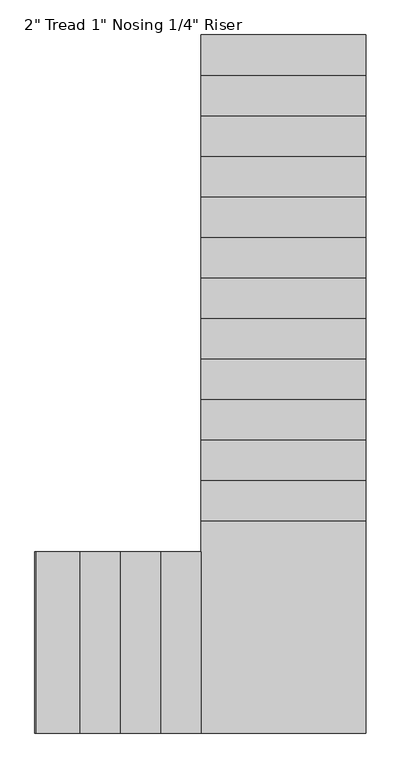
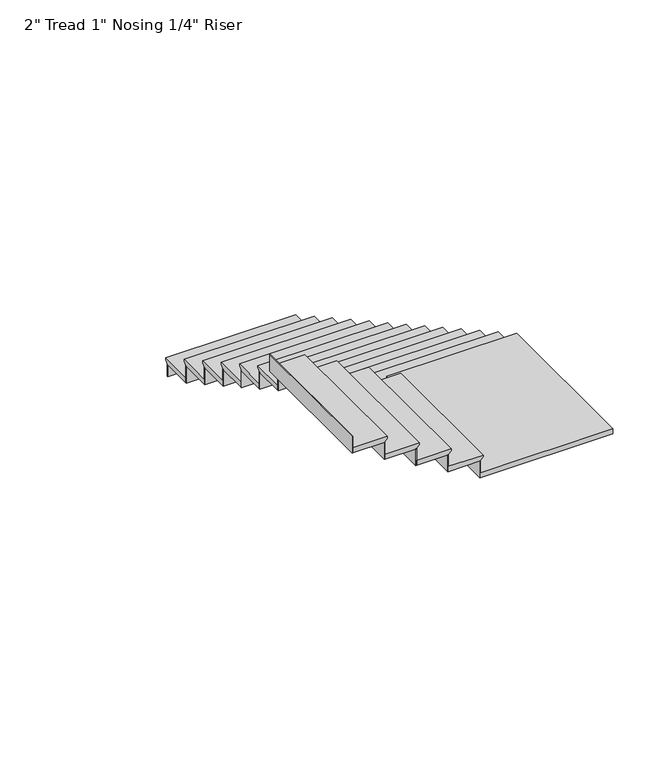
"""IFC4 building model written with IfcOpenShell, lengths in millimetres: stair flight geometry."""

from ifc_helpers import new_model, si_unit, origin, place, context, project, spatial, faceted_brep, source, transform, mapped, element, save


def stair_flight_acf00c5d(model_context):
    return source(origin(), model_context, "Body", "Brep", [
        faceted_brep([(-5006.9237749, -746.7863315, 455.0833333), (-5006.9237749, -746.7863315, 474.1333333), (-3766.7446058, -746.7863315, 474.1333333), (-3766.7446058, -746.7863315, 455.0833333), (-5006.9237749, -772.1863315, 429.6833333), (-3766.7446058, -772.1863315, 429.6833333), (-5006.9237749, -1076.9863315, 474.1333333), (-3766.7446058, -1076.9863315, 474.1333333), (-3766.7446058, -772.1863315, 423.3333333), (-3766.7446058, -1076.9863315, 423.3333333), (-5006.9237749, -1076.9863315, 423.3333333), (-5006.9237749, -772.1863315, 423.3333333)], [[[0, 1, 2, 3]], [[4, 0, 3, 5]], [[2, 1, 6, 7]], [[8, 9, 10, 11]], [[2, 7, 9, 8, 5, 3]], [[8, 11, 4, 5]], [[6, 1, 0, 4, 11, 10]], [[7, 6, 10, 9]]]),
        faceted_brep([(-5006.9237749, -772.1863315, 423.3333333), (-5006.9237749, -772.1863315, 304.8), (-5006.9237749, -778.5363315, 304.8), (-5006.9237749, -778.5363315, 423.3333333), (-3766.7446058, -772.1863315, 423.3333333), (-3766.7446058, -778.5363315, 423.3333333), (-3766.7446058, -778.5363315, 304.8), (-3766.7446058, -772.1863315, 304.8)], [[[0, 1, 2, 3]], [[4, 5, 6, 7]], [[1, 0, 4, 7]], [[2, 1, 7, 6]], [[3, 2, 6, 5]], [[0, 3, 5, 4]]]),
        faceted_brep([(-5006.9237749, -1076.9863315, 592.6666667), (-5006.9237749, -1076.9863315, 423.3333333), (-5006.9237749, -1083.3363315, 423.3333333), (-5006.9237749, -1083.3363315, 592.6666667), (-3766.7446058, -1076.9863315, 592.6666667), (-3766.7446058, -1083.3363315, 592.6666667), (-3766.7446058, -1083.3363315, 423.3333333), (-3766.7446058, -1076.9863315, 423.3333333)], [[[0, 1, 2, 3]], [[4, 5, 6, 7]], [[1, 0, 4, 7]], [[2, 1, 7, 6]], [[3, 2, 6, 5]], [[0, 3, 5, 4]]]),
        faceted_brep([(-3766.7446058, -1051.5863315, 643.4666667), (-5006.9237749, -1051.5863315, 643.4666667), (-5006.9237749, -1381.7863315, 643.4666667), (-3766.7446058, -1381.7863315, 643.4666667), (-3766.7446058, -1076.9863315, 592.6666667), (-3766.7446058, -1381.7863315, 592.6666667), (-5006.9237749, -1381.7863315, 592.6666667), (-5006.9237749, -1076.9863315, 592.6666667), (-3766.7446058, -1076.9863315, 599.0166667), (-3766.7446058, -1051.5863315, 624.4166667), (-5006.9237749, -1076.9863315, 599.0166667), (-5006.9237749, -1051.5863315, 624.4166667)], [[[0, 1, 2, 3]], [[4, 5, 6, 7]], [[0, 3, 5, 4, 8, 9]], [[4, 7, 10, 8]], [[2, 1, 11, 10, 7, 6]], [[3, 2, 6, 5]], [[11, 1, 0, 9]], [[10, 11, 9, 8]]]),
        faceted_brep([(-5006.9237749, -1381.7863315, 762.0), (-5006.9237749, -1381.7863315, 592.6666667), (-5006.9237749, -1388.1363315, 592.6666667), (-5006.9237749, -1388.1363315, 762.0), (-3766.7446058, -1381.7863315, 762.0), (-3766.7446058, -1388.1363315, 762.0), (-3766.7446058, -1388.1363315, 592.6666667), (-3766.7446058, -1381.7863315, 592.6666667)], [[[0, 1, 2, 3]], [[4, 5, 6, 7]], [[1, 0, 4, 7]], [[2, 1, 7, 6]], [[3, 2, 6, 5]], [[0, 3, 5, 4]]]),
        faceted_brep([(-3766.7446058, -1356.3863315, 812.8), (-5006.9237749, -1356.3863315, 812.8), (-5006.9237749, -1686.5863315, 812.8), (-3766.7446058, -1686.5863315, 812.8), (-3766.7446058, -1381.7863315, 762.0), (-3766.7446058, -1686.5863315, 762.0), (-5006.9237749, -1686.5863315, 762.0), (-5006.9237749, -1381.7863315, 762.0), (-3766.7446058, -1381.7863315, 768.35), (-3766.7446058, -1356.3863315, 793.75), (-5006.9237749, -1381.7863315, 768.35), (-5006.9237749, -1356.3863315, 793.75)], [[[0, 1, 2, 3]], [[4, 5, 6, 7]], [[0, 3, 5, 4, 8, 9]], [[4, 7, 10, 8]], [[2, 1, 11, 10, 7, 6]], [[3, 2, 6, 5]], [[11, 1, 0, 9]], [[10, 11, 9, 8]]]),
        faceted_brep([(-5006.9237749, -1686.5863315, 931.3333333), (-5006.9237749, -1686.5863315, 762.0), (-5006.9237749, -1692.9363315, 762.0), (-5006.9237749, -1692.9363315, 931.3333333), (-3766.7446058, -1686.5863315, 931.3333333), (-3766.7446058, -1692.9363315, 931.3333333), (-3766.7446058, -1692.9363315, 762.0), (-3766.7446058, -1686.5863315, 762.0)], [[[0, 1, 2, 3]], [[4, 5, 6, 7]], [[1, 0, 4, 7]], [[2, 1, 7, 6]], [[3, 2, 6, 5]], [[0, 3, 5, 4]]]),
        faceted_brep([(-3766.7446058, -1661.1863315, 982.1333333), (-5006.9237749, -1661.1863315, 982.1333333), (-5006.9237749, -1991.3863315, 982.1333333), (-3766.7446058, -1991.3863315, 982.1333333), (-3766.7446058, -1686.5863315, 931.3333333), (-3766.7446058, -1991.3863315, 931.3333333), (-5006.9237749, -1991.3863315, 931.3333333), (-5006.9237749, -1686.5863315, 931.3333333), (-3766.7446058, -1686.5863315, 937.6833333), (-3766.7446058, -1661.1863315, 963.0833333), (-5006.9237749, -1686.5863315, 937.6833333), (-5006.9237749, -1661.1863315, 963.0833333)], [[[0, 1, 2, 3]], [[4, 5, 6, 7]], [[0, 3, 5, 4, 8, 9]], [[4, 7, 10, 8]], [[2, 1, 11, 10, 7, 6]], [[3, 2, 6, 5]], [[11, 1, 0, 9]], [[10, 11, 9, 8]]]),
        faceted_brep([(-5006.9237749, -1991.3863315, 1100.6666667), (-5006.9237749, -1991.3863315, 931.3333333), (-5006.9237749, -1997.7363315, 931.3333333), (-5006.9237749, -1997.7363315, 1100.6666667), (-3766.7446058, -1991.3863315, 1100.6666667), (-3766.7446058, -1997.7363315, 1100.6666667), (-3766.7446058, -1997.7363315, 931.3333333), (-3766.7446058, -1991.3863315, 931.3333333)], [[[0, 1, 2, 3]], [[4, 5, 6, 7]], [[1, 0, 4, 7]], [[2, 1, 7, 6]], [[3, 2, 6, 5]], [[0, 3, 5, 4]]]),
        faceted_brep([(-3766.7446058, -1965.9863315, 1151.4666667), (-5006.9237749, -1965.9863315, 1151.4666667), (-5006.9237749, -2296.1863315, 1151.4666667), (-3766.7446058, -2296.1863315, 1151.4666667), (-3766.7446058, -1991.3863315, 1100.6666667), (-3766.7446058, -2296.1863315, 1100.6666667), (-5006.9237749, -2296.1863315, 1100.6666667), (-5006.9237749, -1991.3863315, 1100.6666667), (-3766.7446058, -1991.3863315, 1107.0166667), (-3766.7446058, -1965.9863315, 1132.4166667), (-5006.9237749, -1991.3863315, 1107.0166667), (-5006.9237749, -1965.9863315, 1132.4166667)], [[[0, 1, 2, 3]], [[4, 5, 6, 7]], [[0, 3, 5, 4, 8, 9]], [[4, 7, 10, 8]], [[2, 1, 11, 10, 7, 6]], [[3, 2, 6, 5]], [[11, 1, 0, 9]], [[10, 11, 9, 8]]]),
        faceted_brep([(-5006.9237749, -2296.1863315, 1270.0), (-5006.9237749, -2296.1863315, 1100.6666667), (-5006.9237749, -2302.5363315, 1100.6666667), (-5006.9237749, -2302.5363315, 1270.0), (-3766.7446058, -2296.1863315, 1270.0), (-3766.7446058, -2302.5363315, 1270.0), (-3766.7446058, -2302.5363315, 1100.6666667), (-3766.7446058, -2296.1863315, 1100.6666667)], [[[0, 1, 2, 3]], [[4, 5, 6, 7]], [[1, 0, 4, 7]], [[2, 1, 7, 6]], [[3, 2, 6, 5]], [[0, 3, 5, 4]]]),
        faceted_brep([(-3766.7446058, -2270.7863315, 1320.8), (-5006.9237749, -2270.7863315, 1320.8), (-5006.9237749, -2600.9863315, 1320.8), (-3766.7446058, -2600.9863315, 1320.8), (-3766.7446058, -2296.1863315, 1270.0), (-3766.7446058, -2600.9863315, 1270.0), (-5006.9237749, -2600.9863315, 1270.0), (-5006.9237749, -2296.1863315, 1270.0), (-3766.7446058, -2296.1863315, 1276.35), (-3766.7446058, -2270.7863315, 1301.75), (-5006.9237749, -2296.1863315, 1276.35), (-5006.9237749, -2270.7863315, 1301.75)], [[[0, 1, 2, 3]], [[4, 5, 6, 7]], [[0, 3, 5, 4, 8, 9]], [[4, 7, 10, 8]], [[2, 1, 11, 10, 7, 6]], [[3, 2, 6, 5]], [[11, 1, 0, 9]], [[10, 11, 9, 8]]]),
        faceted_brep([(-5006.9237749, -2600.9863315, 1439.3333333), (-5006.9237749, -2600.9863315, 1270.0), (-5006.9237749, -2607.3363315, 1270.0), (-5006.9237749, -2607.3363315, 1439.3333333), (-3766.7446058, -2600.9863315, 1439.3333333), (-3766.7446058, -2607.3363315, 1439.3333333), (-3766.7446058, -2607.3363315, 1270.0), (-3766.7446058, -2600.9863315, 1270.0)], [[[0, 1, 2, 3]], [[4, 5, 6, 7]], [[1, 0, 4, 7]], [[2, 1, 7, 6]], [[3, 2, 6, 5]], [[0, 3, 5, 4]]]),
        faceted_brep([(-3766.7446058, -2575.5863315, 1490.1333333), (-5006.9237749, -2575.5863315, 1490.1333333), (-5006.9237749, -2905.7863315, 1490.1333333), (-3766.7446058, -2905.7863315, 1490.1333333), (-3766.7446058, -2600.9863315, 1439.3333333), (-3766.7446058, -2905.7863315, 1439.3333333), (-5006.9237749, -2905.7863315, 1439.3333333), (-5006.9237749, -2600.9863315, 1439.3333333), (-3766.7446058, -2600.9863315, 1445.6833333), (-3766.7446058, -2575.5863315, 1471.0833333), (-5006.9237749, -2600.9863315, 1445.6833333), (-5006.9237749, -2575.5863315, 1471.0833333)], [[[0, 1, 2, 3]], [[4, 5, 6, 7]], [[0, 3, 5, 4, 8, 9]], [[4, 7, 10, 8]], [[2, 1, 11, 10, 7, 6]], [[3, 2, 6, 5]], [[11, 1, 0, 9]], [[10, 11, 9, 8]]]),
        faceted_brep([(-5006.9237749, -2905.7863315, 1608.6666667), (-5006.9237749, -2905.7863315, 1439.3333333), (-5006.9237749, -2912.1363315, 1439.3333333), (-5006.9237749, -2912.1363315, 1608.6666667), (-3766.7446058, -2905.7863315, 1608.6666667), (-3766.7446058, -2912.1363315, 1608.6666667), (-3766.7446058, -2912.1363315, 1439.3333333), (-3766.7446058, -2905.7863315, 1439.3333333)], [[[0, 1, 2, 3]], [[4, 5, 6, 7]], [[1, 0, 4, 7]], [[2, 1, 7, 6]], [[3, 2, 6, 5]], [[0, 3, 5, 4]]]),
        faceted_brep([(-3766.7446058, -2880.3863315, 1659.4666667), (-5006.9237749, -2880.3863315, 1659.4666667), (-5006.9237749, -3210.5863315, 1659.4666667), (-3766.7446058, -3210.5863315, 1659.4666667), (-3766.7446058, -2905.7863315, 1608.6666667), (-3766.7446058, -3210.5863315, 1608.6666667), (-5006.9237749, -3210.5863315, 1608.6666667), (-5006.9237749, -2905.7863315, 1608.6666667), (-3766.7446058, -2905.7863315, 1615.0166667), (-3766.7446058, -2880.3863315, 1640.4166667), (-5006.9237749, -2905.7863315, 1615.0166667), (-5006.9237749, -2880.3863315, 1640.4166667)], [[[0, 1, 2, 3]], [[4, 5, 6, 7]], [[0, 3, 5, 4, 8, 9]], [[4, 7, 10, 8]], [[2, 1, 11, 10, 7, 6]], [[3, 2, 6, 5]], [[11, 1, 0, 9]], [[10, 11, 9, 8]]]),
        faceted_brep([(-5006.9237749, -3210.5863315, 1778.0), (-5006.9237749, -3210.5863315, 1608.6666667), (-5006.9237749, -3216.9363315, 1608.6666667), (-5006.9237749, -3216.9363315, 1778.0), (-3766.7446058, -3210.5863315, 1778.0), (-3766.7446058, -3216.9363315, 1778.0), (-3766.7446058, -3216.9363315, 1608.6666667), (-3766.7446058, -3210.5863315, 1608.6666667)], [[[0, 1, 2, 3]], [[4, 5, 6, 7]], [[1, 0, 4, 7]], [[2, 1, 7, 6]], [[3, 2, 6, 5]], [[0, 3, 5, 4]]]),
        faceted_brep([(-3766.7446058, -3185.1863315, 1828.8), (-5006.9237749, -3185.1863315, 1828.8), (-5006.9237749, -3515.3863315, 1828.8), (-3766.7446058, -3515.3863315, 1828.8), (-3766.7446058, -3210.5863315, 1778.0), (-3766.7446058, -3515.3863315, 1778.0), (-5006.9237749, -3515.3863315, 1778.0), (-5006.9237749, -3210.5863315, 1778.0), (-3766.7446058, -3210.5863315, 1784.35), (-3766.7446058, -3185.1863315, 1809.75), (-5006.9237749, -3210.5863315, 1784.35), (-5006.9237749, -3185.1863315, 1809.75)], [[[0, 1, 2, 3]], [[4, 5, 6, 7]], [[0, 3, 5, 4, 8, 9]], [[4, 7, 10, 8]], [[2, 1, 11, 10, 7, 6]], [[3, 2, 6, 5]], [[11, 1, 0, 9]], [[10, 11, 9, 8]]]),
        faceted_brep([(-5006.9237749, -3515.3863315, 1947.3333333), (-5006.9237749, -3515.3863315, 1778.0), (-5006.9237749, -3521.7363315, 1778.0), (-5006.9237749, -3521.7363315, 1947.3333333), (-3766.7446058, -3515.3863315, 1947.3333333), (-3766.7446058, -3521.7363315, 1947.3333333), (-3766.7446058, -3521.7363315, 1778.0), (-3766.7446058, -3515.3863315, 1778.0)], [[[0, 1, 2, 3]], [[4, 5, 6, 7]], [[1, 0, 4, 7]], [[2, 1, 7, 6]], [[3, 2, 6, 5]], [[0, 3, 5, 4]]]),
        faceted_brep([(-3766.7446058, -3489.9863315, 1998.1333333), (-5006.9237749, -3489.9863315, 1998.1333333), (-5006.9237749, -3820.1863315, 1998.1333333), (-3766.7446058, -3820.1863315, 1998.1333333), (-3766.7446058, -3515.3863315, 1947.3333333), (-3766.7446058, -3820.1863315, 1947.3333333), (-5006.9237749, -3820.1863315, 1947.3333333), (-5006.9237749, -3515.3863315, 1947.3333333), (-3766.7446058, -3515.3863315, 1953.6833333), (-3766.7446058, -3489.9863315, 1979.0833333), (-5006.9237749, -3515.3863315, 1953.6833333), (-5006.9237749, -3489.9863315, 1979.0833333)], [[[0, 1, 2, 3]], [[4, 5, 6, 7]], [[0, 3, 5, 4, 8, 9]], [[4, 7, 10, 8]], [[2, 1, 11, 10, 7, 6]], [[3, 2, 6, 5]], [[11, 1, 0, 9]], [[10, 11, 9, 8]]]),
        faceted_brep([(-5006.9237749, -3820.1863315, 2116.6666667), (-5006.9237749, -3820.1863315, 1947.3333333), (-5006.9237749, -3826.5363315, 1947.3333333), (-5006.9237749, -3826.5363315, 2116.6666667), (-3766.7446058, -3820.1863315, 2116.6666667), (-3766.7446058, -3826.5363315, 2116.6666667), (-3766.7446058, -3826.5363315, 1947.3333333), (-3766.7446058, -3820.1863315, 1947.3333333)], [[[0, 1, 2, 3]], [[4, 5, 6, 7]], [[1, 0, 4, 7]], [[2, 1, 7, 6]], [[3, 2, 6, 5]], [[0, 3, 5, 4]]]),
        faceted_brep([(-3766.7446058, -3794.7863315, 2167.4666667), (-5006.9237749, -3794.7863315, 2167.4666667), (-5006.9237749, -4124.9863315, 2167.4666667), (-3766.7446058, -4124.9863315, 2167.4666667), (-3766.7446058, -3820.1863315, 2116.6666667), (-3766.7446058, -4124.9863315, 2116.6666667), (-5006.9237749, -4124.9863315, 2116.6666667), (-5006.9237749, -3820.1863315, 2116.6666667), (-3766.7446058, -3820.1863315, 2123.0166667), (-3766.7446058, -3794.7863315, 2148.4166667), (-5006.9237749, -3820.1863315, 2123.0166667), (-5006.9237749, -3794.7863315, 2148.4166667)], [[[0, 1, 2, 3]], [[4, 5, 6, 7]], [[0, 3, 5, 4, 8, 9]], [[4, 7, 10, 8]], [[2, 1, 11, 10, 7, 6]], [[3, 2, 6, 5]], [[11, 1, 0, 9]], [[10, 11, 9, 8]]]),
        faceted_brep([(-5006.9237749, -4124.9863315, 2286.0), (-5006.9237749, -4124.9863315, 2116.6666667), (-5006.9237749, -4131.3363315, 2116.6666667), (-5006.9237749, -4131.3363315, 2286.0), (-3766.7446058, -4124.9863315, 2286.0), (-3766.7446058, -4131.3363315, 2286.0), (-3766.7446058, -4131.3363315, 2116.6666667), (-3766.7446058, -4124.9863315, 2116.6666667)], [[[0, 1, 2, 3]], [[4, 5, 6, 7]], [[1, 0, 4, 7]], [[2, 1, 7, 6]], [[3, 2, 6, 5]], [[0, 3, 5, 4]]]),
        faceted_brep([(-3766.7446058, -4099.5863315, 2336.8), (-5006.9237749, -4099.5863315, 2336.8), (-5006.9237749, -4429.7863315, 2336.8), (-3766.7446058, -4429.7863315, 2336.8), (-3766.7446058, -4124.9863315, 2286.0), (-3766.7446058, -4429.7863315, 2286.0), (-5006.9237749, -4429.7863315, 2286.0), (-5006.9237749, -4124.9863315, 2286.0), (-3766.7446058, -4124.9863315, 2292.35), (-3766.7446058, -4099.5863315, 2317.75), (-5006.9237749, -4124.9863315, 2292.35), (-5006.9237749, -4099.5863315, 2317.75)], [[[0, 1, 2, 3]], [[4, 5, 6, 7]], [[0, 3, 5, 4, 8, 9]], [[4, 7, 10, 8]], [[2, 1, 11, 10, 7, 6]], [[3, 2, 6, 5]], [[11, 1, 0, 9]], [[10, 11, 9, 8]]]),
        faceted_brep([(-5006.9237749, -4429.7863315, 2455.3333333), (-5006.9237749, -4429.7863315, 2286.0), (-5006.9237749, -4436.1363315, 2286.0), (-5006.9237749, -4436.1363315, 2455.3333333), (-3766.7446058, -4429.7863315, 2455.3333333), (-3766.7446058, -4436.1363315, 2455.3333333), (-3766.7446058, -4436.1363315, 2286.0), (-3766.7446058, -4429.7863315, 2286.0)], [[[0, 1, 2, 3]], [[4, 5, 6, 7]], [[1, 0, 4, 7]], [[2, 1, 7, 6]], [[3, 2, 6, 5]], [[0, 3, 5, 4]]]),
        faceted_brep([(-5032.3237749, -5996.1053142, 2506.1333333), (-3766.7446058, -5996.1053142, 2506.1333333), (-3766.7446058, -4404.3863315, 2506.1333333), (-5006.9237749, -4404.3863315, 2506.1333333), (-5006.9237749, -4632.9863315, 2506.1333333), (-5032.3237749, -4632.9863315, 2506.1333333), (-3766.7446058, -5996.1053142, 2455.3333333), (-5032.3237749, -5996.1053142, 2455.3333333), (-5032.3237749, -4632.9863315, 2455.3333333), (-5006.9237749, -4632.9863315, 2455.3333333), (-5006.9237749, -4429.7863315, 2455.3333333), (-3766.7446058, -4429.7863315, 2455.3333333), (-3766.7446058, -4429.7863315, 2461.6833333), (-3766.7446058, -4404.3863315, 2487.0833333), (-5006.9237749, -4429.7863315, 2461.6833333), (-5006.9237749, -4404.3863315, 2487.0833333)], [[[0, 1, 2, 3, 4, 5]], [[6, 7, 8, 9, 10, 11]], [[1, 0, 7, 6]], [[2, 1, 6, 11, 12, 13]], [[11, 10, 14, 12]], [[4, 3, 15, 14, 10, 9]], [[5, 4, 9, 8]], [[0, 5, 8, 7]], [[15, 3, 2, 13]], [[14, 15, 13, 12]]]),
        faceted_brep([(-5032.3237749, -4632.9863315, 2624.6666667), (-5032.3237749, -4632.9863315, 2455.3333333), (-5038.6737749, -4632.9863315, 2455.3333333), (-5038.6737749, -4632.9863315, 2624.6666667), (-5032.3237749, -5996.1053142, 2624.6666667), (-5038.6737749, -5996.1053142, 2624.6666667), (-5038.6737749, -5996.1053142, 2455.3333333), (-5032.3237749, -5996.1053142, 2455.3333333)], [[[0, 1, 2, 3]], [[4, 5, 6, 7]], [[1, 0, 4, 7]], [[2, 1, 7, 6]], [[3, 2, 6, 5]], [[0, 3, 5, 4]]]),
        faceted_brep([(-5006.9237749, -5996.1053142, 2675.4666667), (-5006.9237749, -4632.9863315, 2675.4666667), (-5337.1237749, -4632.9863315, 2675.4666667), (-5337.1237749, -5996.1053142, 2675.4666667), (-5032.3237749, -5996.1053142, 2624.6666667), (-5337.1237749, -5996.1053142, 2624.6666667), (-5337.1237749, -4632.9863315, 2624.6666667), (-5032.3237749, -4632.9863315, 2624.6666667), (-5032.3237749, -5996.1053142, 2631.0166667), (-5006.9237749, -5996.1053142, 2656.4166667), (-5032.3237749, -4632.9863315, 2631.0166667), (-5006.9237749, -4632.9863315, 2656.4166667)], [[[0, 1, 2, 3]], [[4, 5, 6, 7]], [[0, 3, 5, 4, 8, 9]], [[4, 7, 10, 8]], [[2, 1, 11, 10, 7, 6]], [[3, 2, 6, 5]], [[11, 1, 0, 9]], [[10, 11, 9, 8]]]),
        faceted_brep([(-5337.1237749, -4632.9863315, 2794.0), (-5337.1237749, -4632.9863315, 2624.6666667), (-5343.4737749, -4632.9863315, 2624.6666667), (-5343.4737749, -4632.9863315, 2794.0), (-5337.1237749, -5996.1053142, 2794.0), (-5343.4737749, -5996.1053142, 2794.0), (-5343.4737749, -5996.1053142, 2624.6666667), (-5337.1237749, -5996.1053142, 2624.6666667)], [[[0, 1, 2, 3]], [[4, 5, 6, 7]], [[1, 0, 4, 7]], [[2, 1, 7, 6]], [[3, 2, 6, 5]], [[0, 3, 5, 4]]]),
        faceted_brep([(-5311.7237749, -5996.1053142, 2844.8), (-5311.7237749, -4632.9863315, 2844.8), (-5641.9237749, -4632.9863315, 2844.8), (-5641.9237749, -5996.1053142, 2844.8), (-5337.1237749, -5996.1053142, 2794.0), (-5641.9237749, -5996.1053142, 2794.0), (-5641.9237749, -4632.9863315, 2794.0), (-5337.1237749, -4632.9863315, 2794.0), (-5337.1237749, -5996.1053142, 2800.35), (-5311.7237749, -5996.1053142, 2825.75), (-5337.1237749, -4632.9863315, 2800.35), (-5311.7237749, -4632.9863315, 2825.75)], [[[0, 1, 2, 3]], [[4, 5, 6, 7]], [[0, 3, 5, 4, 8, 9]], [[4, 7, 10, 8]], [[2, 1, 11, 10, 7, 6]], [[3, 2, 6, 5]], [[11, 1, 0, 9]], [[10, 11, 9, 8]]]),
        faceted_brep([(-5641.9237749, -4632.9863315, 2963.3333333), (-5641.9237749, -4632.9863315, 2794.0), (-5648.2737749, -4632.9863315, 2794.0), (-5648.2737749, -4632.9863315, 2963.3333333), (-5641.9237749, -5996.1053142, 2963.3333333), (-5648.2737749, -5996.1053142, 2963.3333333), (-5648.2737749, -5996.1053142, 2794.0), (-5641.9237749, -5996.1053142, 2794.0)], [[[0, 1, 2, 3]], [[4, 5, 6, 7]], [[1, 0, 4, 7]], [[2, 1, 7, 6]], [[3, 2, 6, 5]], [[0, 3, 5, 4]]]),
        faceted_brep([(-5616.5237749, -5996.1053142, 3014.1333333), (-5616.5237749, -4632.9863315, 3014.1333333), (-5946.7237749, -4632.9863315, 3014.1333333), (-5946.7237749, -5996.1053142, 3014.1333333), (-5641.9237749, -5996.1053142, 2963.3333333), (-5946.7237749, -5996.1053142, 2963.3333333), (-5946.7237749, -4632.9863315, 2963.3333333), (-5641.9237749, -4632.9863315, 2963.3333333), (-5641.9237749, -5996.1053142, 2969.6833333), (-5616.5237749, -5996.1053142, 2995.0833333), (-5641.9237749, -4632.9863315, 2969.6833333), (-5616.5237749, -4632.9863315, 2995.0833333)], [[[0, 1, 2, 3]], [[4, 5, 6, 7]], [[0, 3, 5, 4, 8, 9]], [[4, 7, 10, 8]], [[2, 1, 11, 10, 7, 6]], [[3, 2, 6, 5]], [[11, 1, 0, 9]], [[10, 11, 9, 8]]]),
        faceted_brep([(-5946.7237749, -4632.9863315, 3132.6666667), (-5946.7237749, -4632.9863315, 2963.3333333), (-5953.0737749, -4632.9863315, 2963.3333333), (-5953.0737749, -4632.9863315, 3132.6666667), (-5946.7237749, -5996.1053142, 3132.6666667), (-5953.0737749, -5996.1053142, 3132.6666667), (-5953.0737749, -5996.1053142, 2963.3333333), (-5946.7237749, -5996.1053142, 2963.3333333)], [[[0, 1, 2, 3]], [[4, 5, 6, 7]], [[1, 0, 4, 7]], [[2, 1, 7, 6]], [[3, 2, 6, 5]], [[0, 3, 5, 4]]]),
        faceted_brep([(-6251.5237749, -4632.9863315, 3302.0), (-6251.5237749, -4632.9863315, 3132.6666667), (-6257.8737749, -4632.9863315, 3132.6666667), (-6257.8737749, -4632.9863315, 3302.0), (-6251.5237749, -5996.1053142, 3302.0), (-6257.8737749, -5996.1053142, 3302.0), (-6257.8737749, -5996.1053142, 3132.6666667), (-6251.5237749, -5996.1053142, 3132.6666667)], [[[0, 1, 2, 3]], [[4, 5, 6, 7]], [[1, 0, 4, 7]], [[2, 1, 7, 6]], [[3, 2, 6, 5]], [[0, 3, 5, 4]]]),
        faceted_brep([(-5921.3237749, -5996.1053142, 3183.4666667), (-5921.3237749, -4632.9863315, 3183.4666667), (-6251.5237749, -4632.9863315, 3183.4666667), (-6251.5237749, -5996.1053142, 3183.4666667), (-5946.7237749, -5996.1053142, 3132.6666667), (-6251.5237749, -5996.1053142, 3132.6666667), (-6251.5237749, -4632.9863315, 3132.6666667), (-5946.7237749, -4632.9863315, 3132.6666667), (-5946.7237749, -5996.1053142, 3139.0166667), (-5921.3237749, -5996.1053142, 3164.4166667), (-5946.7237749, -4632.9863315, 3139.0166667), (-5921.3237749, -4632.9863315, 3164.4166667)], [[[0, 1, 2, 3]], [[4, 5, 6, 7]], [[0, 3, 5, 4, 8, 9]], [[4, 7, 10, 8]], [[2, 1, 11, 10, 7, 6]], [[3, 2, 6, 5]], [[11, 1, 0, 9]], [[10, 11, 9, 8]]]),
    ])


if __name__ == "__main__":
    model = new_model("IFC4")
    model_context = context("Model", 3, world=origin())
    ifc_project = project(units=[si_unit("LENGTHUNIT", "METRE", prefix="MILLI")], contexts=[model_context])
    site = spatial("IfcSite", under=ifc_project)
    building = spatial("IfcBuilding", under=site)
    placement = place(None, origin())
    stair_flight_shape = stair_flight_acf00c5d(model_context)
    element("IfcStairFlight", 1, ObjectType="2\" Tread 1\" Nosing 1/4\" Riser", at=placement, inside=building, context=model_context, shape_type="MappedRepresentation", body=[
        mapped(stair_flight_shape, transform((0.0, 0.0, 0.0), x_axis=(1.0, 0.0, 0.0), y_axis=(0.0, 1.0, 0.0), z_axis=(0.0, 0.0, 1.0))),
    ])
    save(model, "model.ifc")

# Revit data of these elements
# Element 1 (IfcStairFlight, "2\" Tread 1\" Nosing 1/4\" Riser")
#   Materials on its faces: "MARBLE FLOORING 1'"
# Materials
#   "MARBLE FLOORING 1'": class "Generic", colour RGB 120 120 120, transparency 0, Cost = 0
